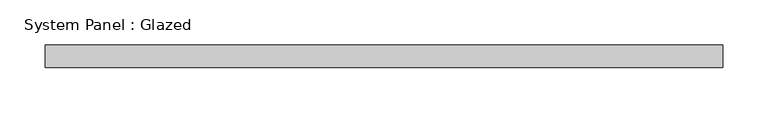
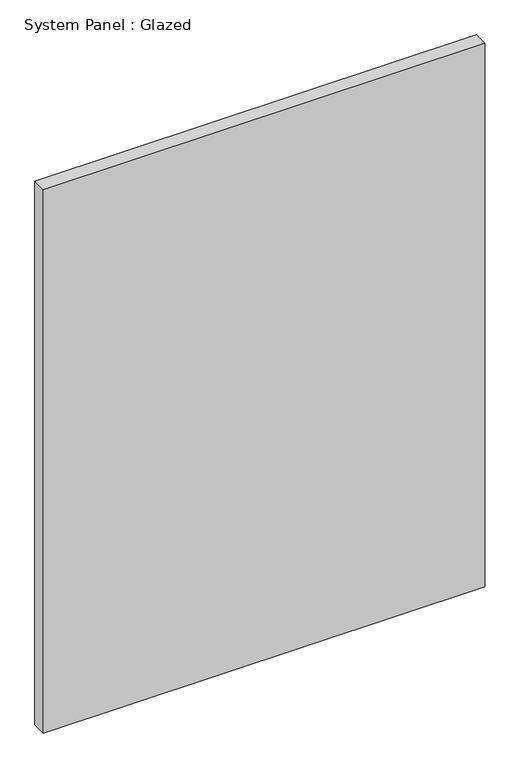
"""IFC4 building model written with IfcOpenShell, lengths in millimetres: plate geometry, System Panel : Glazed."""

from ifc_helpers import new_model, si_unit, origin, origin_with_axes, place, context, project, spatial, polyline, outline, extrude, source, transform, mapped, element, save


def system_panel_glazed_fe2b7919(model_context):
    return source(origin(), model_context, "Body", "SweptSolid", [
        extrude(outline(polyline([(375.0, 24.5), (-375.0, 24.5), (-375.0, 49.5), (375.0, 49.5), (375.0, 24.5)])), origin_with_axes(), (0.0, 0.0, 1.0), 975.0),
    ])


if __name__ == "__main__":
    model = new_model("IFC4")
    model_context = context("Model", 3, world=origin())
    ifc_project = project(units=[si_unit("LENGTHUNIT", "METRE", prefix="MILLI")], contexts=[model_context])
    site = spatial("IfcSite", under=ifc_project)
    building = spatial("IfcBuilding", under=site)
    placement = place(None, origin())
    system_panel_glazed_shape = system_panel_glazed_fe2b7919(model_context)
    element("IfcPlate", 1, ObjectType="System Panel : Glazed", at=placement, inside=building, context=model_context, shape_type="MappedRepresentation", body=[
        mapped(system_panel_glazed_shape, transform((0.0, 0.0, 0.0), x_axis=(1.0, 0.0, 0.0), y_axis=(0.0, 1.0, 0.0), z_axis=(0.0, 0.0, 1.0))),
    ])
    save(model, "model.ifc")

# Revit data of these elements
# Element 1 (IfcPlate, "System Panel : Glazed")
#   Materials on its faces: "Glass"
# Materials
#   "Glass": class "Glass", colour RGB 218 227 224, transparency 0.85, Description = "Soda Lime Glass", Cost = 0
